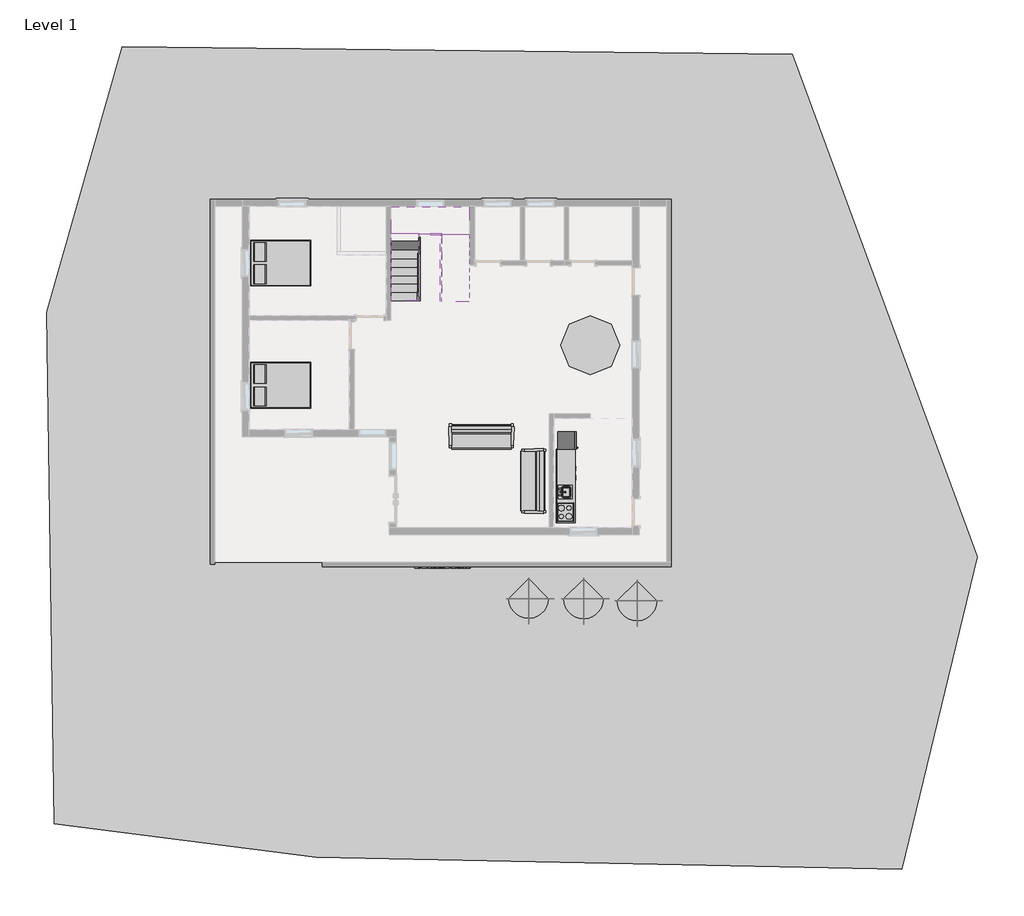
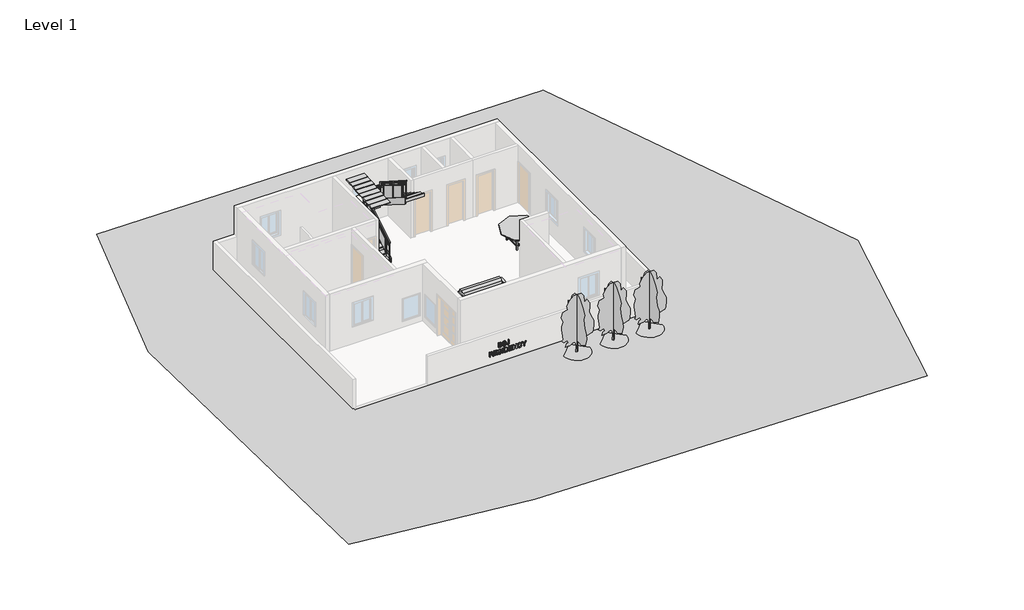
# One storey, part 2 of 2: 6 furniture elements, 6 proxies, 3 geographic elements, 3 members, 3 stair flights, 1 flow terminal, 1 railing, 1 slab.
"""IFC4 building model written with IfcOpenShell, lengths in millimetres."""

from ifc_helpers import new_model, si_unit, frame, origin, place, context, project, spatial, polyline, outline, extrude, faceted_brep, triangles, transform, mapped, element, save
from components import proxy_a6faaae8, proxy_45b28599, kitchenette_medium_kitchenette_medium_844211aa, proxy_c523a7b7, flow_terminal_871c2e40, furniture_1d2926bd, furniture_8d292e24, furniture_aff9b2fb, furniture_7cf74a4d, rpc_tree_deciduous_red_ash_25_5dd3353f, non_monolithic_landing_a2679692, stair_flight_49f3f953, stair_flight_b3fe96e5, stair_flight_42c3951d

model = new_model("IFC4")

# Units and contexts
model_context = context("Model", 3, world=origin())
ifc_project = project(units=[si_unit("LENGTHUNIT", "METRE", prefix="MILLI")], contexts=[model_context])

# Site, building, storey
site = spatial("IfcSite", under=ifc_project)
building = spatial("IfcBuilding", under=site)
storey = spatial("IfcBuildingStorey", under=building, Name="Level 1", Elevation=0.0)

# Proxies
placement = place(None, origin())
element("IfcBuildingElementProxy", 1, Name="Building Element Proxy", at=placement, inside=storey, context=model_context, shape_type="Tessellation", body=[
    triangles([(-16438.8070587, 19561.2664673, -152.4), (5929.6961975, 19305.9913513, -152.4), (12120.1241547, 2521.6364891, -152.4), (9599.2797684, -7912.7437592, -152.4), (-9961.1954681, -7497.921405, -152.4), (-18704.3757477, -6381.0919006, -152.4), (-18959.6520264, 10690.4486298, -152.4)], [[1, 7, 2], [5, 7, 6], [5, 4, 3], [3, 2, 5], [5, 2, 7]], closed=False),
])
element("IfcBuildingElementProxy", 2, Name="24\" Arial", ObjectType="24\" Arial", at=placement, inside=storey, context=model_context, shape_type="SweptSolid", body=[
    extrude(outline(polyline([(834.7006374, -6040.136942), (853.9637739, -6042.7239791), (870.1254059, -6050.4850902), (883.1855332, -6063.4202754), (893.1441559, -6081.5295346), (901.6806431, -6068.3591643), (913.0614012, -6058.9517569), (927.2864302, -6053.3073124), (944.35573, -6051.4258309), (970.4612855, -6056.9085856), (991.2751744, -6073.3568495), (1002.4317716, -6091.8629837), (1006.1506374, -6111.162868), (1006.1506374, -6216.9962013), (765.3210077, -6216.9962013), (765.3210077, -6099.6387939), (770.4362855, -6078.7367106), (785.7821188, -6059.6573124), (808.5950818, -6045.0170346), (834.7006374, -6040.136942)]), holes=[polyline([(939.8872114, -6081.411942), (925.0852438, -6084.4987476), (913.3700818, -6093.7591643), (906.7554985, -6105.3567337), (904.5506374, -6118.7475902), (904.5506374, -6186.8924976), (979.8098966, -6186.8924976), (979.8098966, -6131.7415717), (977.5168411, -6113.6176133), (970.6376744, -6098.2864791), (957.3938087, -6085.6305763), (939.8872114, -6081.411942)]), polyline([(835.6413781, -6070.2406457), (818.6786466, -6072.9232268), (804.4793411, -6080.9709698), (794.8661466, -6092.9139675), (791.6617485, -6107.2823124), (791.6617485, -6186.8924976), (878.2098966, -6186.8924976), (878.2098966, -6118.9827754), (875.5493642, -6097.6580937), (867.567767, -6082.4261782), (854.265105, -6073.2870288), (835.6413781, -6070.2406457)])]), frame((0.0, 2146.5230289, 0.0), z_axis=(0.0, 1.0, 0.0), x_axis=(0.0, 0.0, 1.0)), (0.0, 0.0, 1.0), 50.8),
    extrude(outline(polyline([(834.4066559, -5829.4110161), (854.1034151, -5832.4978217), (871.5659151, -5841.7582383), (884.427605, -5855.4136782), (892.0858225, -5872.3911087), (911.4886003, -5946.1216643), (916.4679117, -5959.2663113), (923.3507531, -5968.6553448), (932.1371246, -5974.288765), (942.8270262, -5976.1665717), (958.8343179, -5972.352162), (971.9311929, -5960.9089328), (980.6624429, -5943.9241527), (983.5728596, -5923.4850902), (980.8241327, -5900.436942), (972.5779522, -5882.6804606), (957.3056142, -5869.6129837), (936.0654522, -5864.3948124), (936.0654522, -5835.8198124), (966.7277207, -5842.12939), (978.7736119, -5849.3990008), (988.6293411, -5859.4118263), (1001.7703133, -5887.6671214), (1006.1506374, -5926.8952754), (1001.4763318, -5959.0862476), (987.4534151, -5984.3980532), (965.8310772, -6000.8022198), (938.3585077, -6006.2702754), (919.0145262, -6003.2790138), (903.4335077, -5994.3052291), (891.6154522, -5979.3489212), (883.5603596, -5958.4100902), (866.6858225, -5894.3221272), (861.1111987, -5879.0938865), (853.5007531, -5868.2165717), (843.8544857, -5861.6901828), (832.1723966, -5859.5147198), (814.4379637, -5863.3658772), (800.2754059, -5874.9193495), (790.9929406, -5892.7052291), (787.8987855, -5915.2536087), (791.2281258, -5945.7027407), (801.2161466, -5966.9649513), (818.5243063, -5980.0397777), (843.8140633, -5985.9267569), (843.8140633, -6013.7962013), (810.5574082, -6007.5196967), (797.1206171, -6000.1591353), (785.811517, -5989.9837013), (776.8469192, -5977.0742395), (770.443635, -5961.5115948), (765.3210077, -5922.4267569), (770.0908573, -5884.451699), (784.4004059, -5854.8404143), (794.6805708, -5843.7150526), (806.4416675, -5835.7683657), (819.6836958, -5831.0003535), (834.4066559, -5829.4110161)])), frame((0.0, 2146.5230289, 0.0), z_axis=(0.0, 1.0, 0.0), x_axis=(0.0, 0.0, 1.0)), (0.0, 0.0, 1.0), 50.8),
    extrude(outline(polyline([(823.70573, -5675.1295346), (1006.1506374, -5675.1295346), (1006.1506374, -5705.2332383), (833.0543411, -5705.2332383), (815.6432878, -5707.9011203), (802.5684614, -5715.9047661), (794.3884267, -5728.1123471), (791.6617485, -5743.3920346), (794.0944452, -5756.8563865), (801.3925355, -5767.4985161), (812.6593758, -5774.42178), (826.9983225, -5776.7295346), (848.1061929, -5776.7295346), (848.1061929, -5806.8332383), (821.3538781, -5806.8332383), (800.5105911, -5802.805692), (782.9011003, -5790.7230532), (769.7160309, -5769.6298819), (765.3210077, -5742.4512939), (766.8056142, -5725.7751944), (771.2594337, -5711.2010624), (778.6824661, -5698.7288981), (789.0747114, -5688.3587013), (806.052142, -5678.4368263), (823.70573, -5675.1295346)])), frame((0.0, 2146.5230289, 0.0), z_axis=(0.0, 1.0, 0.0), x_axis=(0.0, 0.0, 1.0)), (0.0, 0.0, 1.0), 50.8),
    extrude(outline(polyline([(407.8395262, -6475.1707383), (415.7770262, -6475.1707383), (424.861054, -6482.3144883), (436.2381374, -6485.5188865), (486.4501744, -6487.9295346), (507.6168411, -6493.2799976), (526.7844337, -6514.9758309), (538.5730911, -6501.49678), (551.4788781, -6491.8688865), (565.5017948, -6486.0921504), (580.6418411, -6484.1665717), (609.4373272, -6487.811942), (629.8543411, -6498.7480532), (638.0858225, -6508.8058946), (643.9654522, -6521.8109004), (648.6691559, -6556.662405), (648.6691559, -6664.7887939), (407.8395262, -6664.7887939), (407.8395262, -6634.6850902), (513.2024892, -6634.6850902), (513.2024892, -6554.8397198), (510.4243642, -6539.2219536), (502.0899892, -6527.881618), (488.1993642, -6520.8187129), (468.7524892, -6518.0332383), (430.7112855, -6517.0924976), (407.8395262, -6511.3304606), (407.8395262, -6475.1707383)]), holes=[polyline([(585.58073, -6514.2702754), (565.4393237, -6516.8132152), (551.052605, -6524.4420346), (542.4205737, -6537.1567337), (539.54323, -6554.9573124), (539.54323, -6634.6850902), (622.3284151, -6634.6850902), (622.3284151, -6555.2512939), (619.8883688, -6538.7368842), (612.56823, -6525.6473587), (600.9412624, -6517.1145462), (585.58073, -6514.2702754)])]), frame((0.0, 2146.5230289, 0.0), z_axis=(0.0, 1.0, 0.0), x_axis=(0.0, 0.0, 1.0)), (0.0, 0.0, 1.0), 50.8),
    extrude(outline(polyline([(407.8395262, -6265.9735161), (434.180267, -6265.9735161), (434.180267, -6405.1443495), (520.7284151, -6405.1443495), (520.7284151, -6276.674442), (547.0691559, -6276.674442), (547.0691559, -6405.1443495), (622.3284151, -6405.1443495), (622.3284151, -6271.500368), (648.6691559, -6271.500368), (648.6691559, -6435.2480532), (407.8395262, -6435.2480532), (407.8395262, -6265.9735161)])), frame((0.0, 2146.5230289, 0.0), z_axis=(0.0, 1.0, 0.0), x_axis=(0.0, 0.0, 1.0)), (0.0, 0.0, 1.0), 50.8),
    extrude(outline(polyline([(476.9251744, -6047.662868), (496.6219337, -6050.7496735), (514.0844337, -6060.0100902), (526.9461235, -6073.66553), (534.6043411, -6090.6429606), (554.0071188, -6164.3735161), (558.9864302, -6177.5181631), (565.8692716, -6186.9071967), (574.6556431, -6192.5406168), (585.3455448, -6194.4184235), (601.3528364, -6190.6040138), (614.4497114, -6179.1607846), (623.1809614, -6162.1760045), (626.0913781, -6141.736942), (623.3426512, -6118.6887939), (615.0964707, -6100.9323124), (599.8241327, -6087.8648356), (578.5839707, -6082.6466643), (578.5839707, -6054.0716643), (609.2462392, -6060.3812418), (621.2921304, -6067.6508526), (631.1478596, -6077.6636782), (644.2888318, -6105.9189733), (648.6691559, -6145.1471272), (643.9948503, -6177.3380995), (629.9719337, -6202.649905), (608.3495957, -6219.0540717), (580.8770262, -6224.5221272), (561.5330448, -6221.5308657), (545.9520262, -6212.5570809), (534.1339707, -6197.6007731), (526.0788781, -6176.661942), (509.2043411, -6112.5739791), (503.6297172, -6097.3457383), (496.0192716, -6086.4684235), (486.3730043, -6079.9420346), (474.6909151, -6077.7665717), (456.9564823, -6081.6177291), (442.7939244, -6093.1712013), (433.5114591, -6110.9570809), (430.417304, -6133.5054606), (433.7466443, -6163.9545925), (443.7346651, -6185.2168032), (461.0428249, -6198.2916295), (486.3325818, -6204.1786087), (486.3325818, -6232.0480532), (453.0759267, -6225.7715485), (439.6391356, -6218.4109872), (428.3300355, -6208.2355532), (419.3654377, -6195.3260913), (412.9621536, -6179.7634467), (407.8395262, -6140.6786087), (412.6093758, -6102.7035508), (426.9189244, -6073.0922661), (437.1990893, -6061.9669044), (448.960186, -6054.0202175), (462.2022143, -6049.2522054), (476.9251744, -6047.662868)])), frame((0.0, 2146.5230289, 0.0), z_axis=(0.0, 1.0, 0.0), x_axis=(0.0, 0.0, 1.0)), (0.0, 0.0, 1.0), 50.8),
    extrude(outline(polyline([(-5972.4036087, 2146.5230289), (-6002.5073124, 2146.5230289), (-6002.5073124, 2197.3230289), (-5972.4036087, 2197.3230289), (-5972.4036087, 2146.5230289)])), frame((0.0, 0.0, 407.8395262), z_axis=(0.0, 0.0, 1.0), x_axis=(1.0, 0.0, 0.0)), (0.0, 0.0, 1.0), 240.8296296),
    extrude(outline(polyline([(530.429804, -5727.8110161), (558.3286466, -5729.8247893), (582.9348966, -5735.8661087), (604.248554, -5745.9349745), (622.2696188, -5760.0313865), (633.8194163, -5773.5214617), (642.0692716, -5787.9449282), (647.0191848, -5803.3017858), (648.6691559, -5819.5920346), (648.6691559, -5915.9591643), (407.8395262, -5915.9591643), (407.8395262, -5812.4188865), (409.8202265, -5797.3045636), (415.7623272, -5782.8884467), (425.6658283, -5769.1705358), (439.53073, -5756.1508309), (458.7277207, -5743.752162), (480.2765633, -5734.8959698), (504.1772577, -5729.5822545), (530.429804, -5727.8110161)]), holes=[polyline([(530.429804, -5757.9147198), (491.5801512, -5761.6923819), (461.2265633, -5773.025368), (449.3938087, -5781.6169768), (440.9418411, -5791.693192), (435.8706605, -5803.2540138), (434.180267, -5816.299442), (434.180267, -5885.8554606), (622.3284151, -5885.8554606), (622.3284151, -5824.5309235), (616.5663781, -5797.2053448), (609.3638318, -5785.9348298), (599.280267, -5776.2591643), (569.8674198, -5762.5008309), (530.429804, -5757.9147198)])]), frame((0.0, 2146.5230289, 0.0), z_axis=(0.0, 1.0, 0.0), x_axis=(0.0, 0.0, 1.0)), (0.0, 0.0, 1.0), 50.8),
    extrude(outline(polyline([(407.8395262, -5513.3809235), (434.180267, -5513.3809235), (434.180267, -5652.5517569), (520.7284151, -5652.5517569), (520.7284151, -5524.0818495), (547.0691559, -5524.0818495), (547.0691559, -5652.5517569), (622.3284151, -5652.5517569), (622.3284151, -5518.9077754), (648.6691559, -5518.9077754), (648.6691559, -5682.6554606), (407.8395262, -5682.6554606), (407.8395262, -5513.3809235)])), frame((0.0, 2146.5230289, 0.0), z_axis=(0.0, 1.0, 0.0), x_axis=(0.0, 0.0, 1.0)), (0.0, 0.0, 1.0), 50.8),
    extrude(outline(polyline([(407.8395262, -5287.5443495), (648.6691559, -5287.5443495), (648.6691559, -5317.6480532), (457.5811929, -5317.6480532), (648.6691559, -5432.4772198), (648.6691559, -5471.9295346), (407.8395262, -5471.9295346), (407.8395262, -5441.8258309), (599.9270262, -5441.8258309), (407.8395262, -5322.0577754), (407.8395262, -5287.5443495)])), frame((0.0, 2146.5230289, 0.0), z_axis=(0.0, 1.0, 0.0), x_axis=(0.0, 0.0, 1.0)), (0.0, 0.0, 1.0), 50.8),
    extrude(outline(polyline([(498.0330448, -5042.2462013), (498.0330448, -5073.4670346), (470.0974545, -5083.7784351), (450.1434614, -5098.7200439), (438.1710656, -5118.291861), (434.180267, -5142.4938865), (435.7879782, -5158.1447256), (440.6111119, -5172.2301133), (448.649668, -5184.7500497), (459.9036466, -5195.7045346), (489.3826397, -5210.9621735), (526.3728596, -5216.0480532), (565.5973387, -5211.0871157), (581.951896, -5204.8859438), (596.1346651, -5196.2043032), (607.5944308, -5185.4684669), (615.7799776, -5173.1047082), (620.6913058, -5159.1130271), (622.3284151, -5143.4934235), (619.3518526, -5122.4847719), (610.4221651, -5104.7319652), (595.5393526, -5090.2350034), (574.7034151, -5078.9938865), (574.7034151, -5047.1262939), (606.4754637, -5062.3104374), (629.7073503, -5083.8739791), (643.9287045, -5110.6850902), (648.6691559, -5141.611942), (646.3981489, -5165.3362476), (639.5851281, -5186.3559235), (628.2300934, -5204.6709698), (612.3330448, -5220.2813865), (594.6022867, -5231.5996735), (574.6299198, -5239.6841643), (552.4159441, -5244.5348587), (527.9603596, -5246.1517569), (502.2314678, -5244.3621446), (479.137385, -5238.9933078), (458.6781113, -5230.0452464), (440.8536466, -5217.5179606), (426.409969, -5202.0545346), (416.0930563, -5184.2980532), (409.9029088, -5164.2485161), (407.8395262, -5141.9059235), (413.4766212, -5106.4407326), (420.5229898, -5091.3457022), (430.3879059, -5078.0090485), (458.5733804, -5056.6108714), (498.0330448, -5042.2462013)])), frame((0.0, 2146.5230289, 0.0), z_axis=(0.0, 1.0, 0.0), x_axis=(0.0, 0.0, 1.0)), (0.0, 0.0, 1.0), 50.8),
    extrude(outline(polyline([(648.6691559, -4814.4693495), (648.6691559, -4849.8059235), (531.4881374, -4917.774442), (648.6691559, -4986.624905), (648.6691559, -5024.136942), (502.3251744, -4933.8258309), (407.8395262, -4933.8258309), (407.8395262, -4903.7221272), (504.1478596, -4903.7221272), (648.6691559, -4814.4693495)])), frame((0.0, 2146.5230289, 0.0), z_axis=(0.0, 1.0, 0.0), x_axis=(0.0, 0.0, 1.0)), (0.0, 0.0, 1.0), 50.8),
])
proxy_shape = proxy_a6faaae8(model_context)
element("IfcBuildingElementProxy", 3, Name="Cook Top-4 Unit2 : 22\" x 20\"", ObjectType="Cook Top-4 Unit2 : 22\" x 20\"", at=placement, inside=storey, context=model_context, shape_type="MappedRepresentation", body=[
    mapped(proxy_shape, transform((-1644.6867944, 4013.4230289, 0.0), x_axis=(0.0, 1.0000000000000009, 0.0), y_axis=(-1.0000000000000009, 0.0, 0.0), z_axis=(0.0, 0.0, 1.0))),
])
proxy_2_shape = proxy_45b28599(model_context)
element("IfcBuildingElementProxy", 4, Name="Dishwasher : 24\" x 24\" x 34\"", ObjectType="Dishwasher : 24\" x 24\" x 34\"", at=placement, inside=storey, context=model_context, shape_type="MappedRepresentation", body=[
    mapped(proxy_2_shape, transform((-1352.8372296, 4964.6055604, 0.0), x_axis=(0.0, 1.0000000000000009, 0.0), y_axis=(-1.0000000000000009, 0.0, 0.0), z_axis=(0.0, 0.0, 1.0))),
])
kitchenette_medium_kitchenette_medium_shape = kitchenette_medium_kitchenette_medium_844211aa(model_context)
element("IfcBuildingElementProxy", 5, Name="Kitchenette - Medium : Kitchenette - Medium", ObjectType="Kitchenette - Medium : Kitchenette - Medium", at=placement, inside=storey, context=model_context, shape_type="MappedRepresentation", body=[
    mapped(kitchenette_medium_kitchenette_medium_shape, transform((-1949.4867944, 4337.585324, 0.0), x_axis=(0.0, 1.0000000000000009, 0.0), y_axis=(-1.0000000000000009, 0.0, 0.0), z_axis=(0.0, 0.0, 1.0))),
])
proxy_3_shape = proxy_c523a7b7(model_context)
element("IfcBuildingElementProxy", 6, Name="Refrigerator : 24\" x 25\" LH", ObjectType="Refrigerator : 24\" x 25\" LH", at=placement, inside=storey, context=model_context, shape_type="MappedRepresentation", body=[
    mapped(proxy_3_shape, transform((-1599.0378229, 6407.3730289, 0.0), x_axis=(0.0, 1.0000000000000009, 0.0), y_axis=(-1.0000000000000009, 0.0, 0.0), z_axis=(0.0, 0.0, 1.0))),
])

# Flow terminal
flow_terminal_shape = flow_terminal_871c2e40(model_context)
element("IfcFlowTerminal", 7, ObjectType="Sink Kitchen-Island : 18\" x 18\"", at=placement, inside=storey, context=model_context, shape_type="MappedRepresentation", body=[
    mapped(flow_terminal_shape, transform((-1642.3413933, 4670.8337884, -14.4), x_axis=(0.0, 1.0000000000000009, 0.0), y_axis=(-1.0000000000000009, 0.0, 0.0), z_axis=(0.0, 0.0, 1.0))),
])

# Furniture
furniture_shape = furniture_1d2926bd(model_context)
element("IfcFurniture", 8, ObjectType="Bed-Box : Queen 60\" x 79\"", at=placement, inside=storey, context=model_context, shape_type="MappedRepresentation", body=[
    mapped(furniture_shape, transform((-11378.7163026, 7916.0705699, 0.0), x_axis=(0.0, 1.0000000000000002, 0.0), y_axis=(-1.0000000000000002, 0.0, 0.0), z_axis=(0.0, 0.0, 1.0))),
])
element("IfcFurniture", 9, ObjectType="Bed-Box : Queen 60\" x 79\"", at=placement, inside=storey, context=model_context, shape_type="MappedRepresentation", body=[
    mapped(furniture_shape, transform((-11378.7163026, 11992.7705699, 0.0), x_axis=(0.0, 1.0000000000000002, 0.0), y_axis=(-1.0000000000000002, 0.0, 0.0), z_axis=(0.0, 0.0, 1.0))),
])
furniture_2_shape = furniture_8d292e24(model_context)
element("IfcFurniture", 10, ObjectType="Counter Top w Sink Hole : 24\" Depth", at=placement, inside=storey, context=model_context, shape_type="MappedRepresentation", body=[
    mapped(furniture_2_shape, transform((-1949.4867944, 4870.985324, -14.4), x_axis=(0.0, 1.0000000000000009, 0.0), y_axis=(-1.0000000000000009, 0.0, 0.0), z_axis=(0.0, 0.0, 1.0))),
])
furniture_3_shape = furniture_aff9b2fb(model_context)
element("IfcFurniture", 11, ObjectType="Sofa-Pensi : 84\"", at=placement, inside=storey, context=model_context, shape_type="MappedRepresentation", body=[
    mapped(furniture_3_shape, transform((-4719.9800439, 6263.6131929, 0.0), x_axis=(1.0, 0.0, 0.0), y_axis=(0.0, 1.0, 0.0), z_axis=(0.0, 0.0, 1.0))),
])
element("IfcFurniture", 12, ObjectType="Sofa-Pensi : 84\"", at=placement, inside=storey, context=model_context, shape_type="MappedRepresentation", body=[
    mapped(furniture_3_shape, transform((-2988.5966305, 5333.4292789, 0.0), x_axis=(0.0, -1.0000000000000002, 0.0), y_axis=(1.0000000000000002, 0.0, 0.0), z_axis=(0.0, 0.0, 1.0))),
])
furniture_4_shape = furniture_7cf74a4d(model_context)
element("IfcFurniture", 13, ObjectType="Table-Dining Round w Chairs : 60\" Diameter", at=placement, inside=storey, context=model_context, shape_type="MappedRepresentation", body=[
    mapped(furniture_4_shape, transform((-910.1687616, 9773.6017175, 0.0), x_axis=(1.0, 0.0, 0.0), y_axis=(0.0, 1.0, 0.0), z_axis=(0.0, 0.0, 1.0))),
])

# Geographic elements
rpc_tree_deciduous_red_ash_25_shape = rpc_tree_deciduous_red_ash_25_5dd3353f(model_context)
element("IfcGeographicElement", 14, ObjectType="RPC Tree - Deciduous : Red Ash - 25'", at=placement, inside=storey, context=model_context, shape_type="MappedRepresentation", body=[
    mapped(rpc_tree_deciduous_red_ash_25_shape, transform((-2863.8867944, 1130.5230289, 0.0), x_axis=(1.0, 0.0, 0.0), y_axis=(0.0, 1.0, 0.0), z_axis=(0.0, 0.0, 1.0))),
])
element("IfcGeographicElement", 15, ObjectType="RPC Tree - Deciduous : Red Ash - 25'", at=placement, inside=storey, context=model_context, shape_type="MappedRepresentation", body=[
    mapped(rpc_tree_deciduous_red_ash_25_shape, transform((755.6132056, 1054.3230289, 0.0), x_axis=(1.0, 0.0, 0.0), y_axis=(0.0, 1.0, 0.0), z_axis=(0.0, 0.0, 1.0))),
])
element("IfcGeographicElement", 16, ObjectType="RPC Tree - Deciduous : Red Ash - 25'", at=placement, inside=storey, context=model_context, shape_type="MappedRepresentation", body=[
    mapped(rpc_tree_deciduous_red_ash_25_shape, transform((-1030.0266382, 1118.9211458, 0.0), x_axis=(1.0, 0.0, 0.0), y_axis=(0.0, 1.0, 0.0), z_axis=(0.0, 0.0, 1.0))),
])

# Members
element("IfcMember", 17, ObjectType="Stringer - 2\" Width", at=placement, inside=storey, context=model_context, shape_type="SweptSolid", body=[
    extrude(outline(polyline([(11074.6230289, 0.0), (11074.6230289, 215.0106437), (13259.0230289, 1605.083371), (13259.0230289, 1243.8010268), (11304.4785583, 0.0), (11074.6230289, 0.0)])), frame((-6534.1867944, 0.0, 0.0), z_axis=(1.0, 0.0, 0.0), x_axis=(0.0, 1.0, 0.0)), (0.0, 0.0, 1.0), 50.8),
])
element("IfcMember", 18, ObjectType="Stringer - 2\" Width", at=placement, inside=storey, context=model_context, shape_type="SweptSolid", body=[
    extrude(outline(polyline([(13259.0230289, 1841.3136224), (13259.0230289, 1480.0312782), (11064.8419954, 2876.3282995), (11064.8419954, 3237.6106437), (13259.0230289, 1841.3136224)])), frame((-5812.9737939, 0.0, 0.0), z_axis=(1.0, 0.0, 0.0), x_axis=(0.0, 1.0, 0.0)), (0.0, 0.0, 1.0), 50.8),
])
element("IfcMember", 19, ObjectType="Stringer - 2\" Width", at=placement, inside=storey, context=model_context, shape_type="SweptSolid", body=[
    extrude(outline(polyline([(-6534.1867944, 13259.0230289), (-6534.1867944, 13309.8230289), (-5762.1737939, 13309.8230289), (-5762.1737939, 13259.0230289), (-6534.1867944, 13259.0230289)])), frame((0.0, 0.0, 1371.6), z_axis=(0.0, 0.0, 1.0), x_axis=(1.0, 0.0, 0.0)), (0.0, 0.0, 1.0), 304.8),
])

# Railing
element("IfcRailing", 20, ObjectType="Glass Panel - Bottom Fill", at=placement, inside=storey, context=model_context, shape_type="SolidModel", body=[
    faceted_brep([(-6584.9867944, 11074.6230289, 1092.2), (-6584.9867944, 11074.6230289, 1031.986276), (-6534.1867944, 11074.6230289, 1031.986276), (-6534.1867944, 11074.6230289, 1092.2), (-5711.3737939, 11064.8419954, 4114.8), (-5762.1737939, 11064.8419954, 4114.8), (-5762.1737939, 11064.8419954, 4054.586276), (-5711.3737939, 11064.8419954, 4054.586276), (-6534.1867944, 13284.4230289, 2438.2226396), (-6534.1867944, 13233.6230289, 2466.1090909), (-6584.9867944, 13233.6230289, 2466.1090909), (-6457.9867944, 13309.8230289, 2514.6), (-6457.9867944, 13309.8230289, 2463.8), (-5762.1737939, 13309.8230289, 2463.8), (-5762.1737939, 13309.8230289, 2514.6), (-6457.9867944, 13360.6230289, 2514.6), (-5711.3737939, 13360.6230289, 2514.6), (-5762.1737939, 13300.0419954, 2692.4), (-5762.1737939, 13249.2419954, 2664.5135487), (-5711.3737939, 13300.0419954, 2692.4), (-6584.9867944, 13284.4230289, 2438.2226396), (-6584.9867944, 13233.6230289, 2514.6), (-6584.9867944, 13284.4230289, 2463.8), (-6534.1867944, 13284.4230289, 2463.8), (-6534.1867944, 13233.6230289, 2514.6), (-6584.9867944, 13360.6230289, 2514.6), (-6584.9867944, 13360.6230289, 2463.8), (-6534.1867944, 13309.8230289, 2463.8), (-6534.1867944, 13309.8230289, 2514.6), (-6457.9867944, 13360.6230289, 2463.8), (-5711.3737939, 13360.6230289, 2463.8), (-5711.3737939, 13300.0419954, 2514.6), (-5711.3737939, 13249.2419954, 2463.8), (-5762.1737939, 13249.2419954, 2463.8), (-5762.1737939, 13300.0419954, 2514.6), (-5711.3737939, 13249.2419954, 2664.5135487)], [[[0, 1, 2, 3]], [[4, 5, 6, 7]], [[3, 2, 8, 9]], [[0, 3, 9, 10]], [[11, 12, 13, 14]], [[15, 11, 14, 16]], [[17, 18, 6, 5]], [[19, 17, 5, 4]], [[1, 0, 10, 20]], [[2, 1, 20, 8]], [[20, 10, 21, 22]], [[8, 20, 22, 23]], [[9, 8, 23, 24]], [[10, 9, 24, 21]], [[22, 21, 25, 26]], [[23, 22, 26, 27]], [[24, 23, 27, 28]], [[21, 24, 28, 25]], [[26, 25, 15, 29]], [[27, 26, 29, 12]], [[28, 27, 12, 11]], [[25, 28, 11, 15]], [[29, 15, 16, 30]], [[12, 29, 30, 13]], [[30, 16, 31, 32]], [[13, 30, 32, 33]], [[14, 13, 33, 34]], [[16, 14, 34, 31]], [[32, 31, 19, 35]], [[33, 32, 35, 18]], [[34, 33, 18, 17]], [[31, 34, 17, 19]], [[35, 19, 4, 7]], [[18, 35, 7, 6]]]),
    faceted_brep([(-6546.8867944, 11074.6230289, 1005.653431), (-6572.2867944, 11074.6230289, 1005.653431), (-6572.2867944, 11074.6230289, 975.546569), (-6546.8867944, 11074.6230289, 975.546569), (-6546.8867944, 13317.6902093, 2433.0598185), (-6546.8867944, 13331.3268468, 2411.6308167), (-6572.2867944, 13352.7558486, 2425.2674542), (-6572.2867944, 13339.1192111, 2446.696456)], [[[0, 1, 2, 3]], [[4, 5, 6, 7]], [[1, 0, 4, 7]], [[2, 1, 7, 6]], [[3, 2, 6, 5]], [[0, 3, 5, 4]]]),
    faceted_brep([(-6555.6906123, 13322.5230289, 2425.7), (-6577.1196141, 13347.9230289, 2425.7), (-6563.4829766, 13347.9230289, 2400.3), (-6542.0539748, 13322.5230289, 2400.3), (-5749.4737939, 13322.5230289, 2425.7), (-5749.4737939, 13322.5230289, 2400.3), (-5724.0737939, 13347.9230289, 2400.3), (-5724.0737939, 13347.9230289, 2425.7)], [[[0, 1, 2, 3]], [[4, 5, 6, 7]], [[1, 0, 4, 7]], [[2, 1, 7, 6]], [[3, 2, 6, 5]], [[0, 3, 5, 4]]]),
    faceted_brep([(-5749.4737939, 13303.7402441, 2603.5), (-5724.0737939, 13303.7402441, 2603.5), (-5724.0737939, 13296.3437467, 2578.1), (-5749.4737939, 13296.3437467, 2578.1), (-5749.4737939, 11064.8419954, 4028.253431), (-5749.4737939, 11064.8419954, 3998.146569), (-5724.0737939, 11064.8419954, 3998.146569), (-5724.0737939, 11064.8419954, 4028.253431)], [[[0, 1, 2, 3]], [[4, 5, 6, 7]], [[1, 0, 4, 7]], [[2, 1, 7, 6]], [[3, 2, 6, 5]], [[0, 3, 5, 4]]]),
    faceted_brep([(-6546.8867944, 11074.6230289, 904.053431), (-6572.2867944, 11074.6230289, 904.053431), (-6572.2867944, 11074.6230289, 873.946569), (-6546.8867944, 11074.6230289, 873.946569), (-6546.8867944, 13317.6902093, 2331.4598185), (-6546.8867944, 13331.3268468, 2310.0308167), (-6572.2867944, 13352.7558486, 2323.6674542), (-6572.2867944, 13339.1192111, 2345.096456)], [[[0, 1, 2, 3]], [[4, 5, 6, 7]], [[1, 0, 4, 7]], [[2, 1, 7, 6]], [[3, 2, 6, 5]], [[0, 3, 5, 4]]]),
    faceted_brep([(-6555.6906123, 13322.5230289, 2324.1), (-6577.1196141, 13347.9230289, 2324.1), (-6563.4829766, 13347.9230289, 2298.7), (-6542.0539748, 13322.5230289, 2298.7), (-5749.4737939, 13322.5230289, 2324.1), (-5749.4737939, 13322.5230289, 2298.7), (-5724.0737939, 13347.9230289, 2298.7), (-5724.0737939, 13347.9230289, 2324.1)], [[[0, 1, 2, 3]], [[4, 5, 6, 7]], [[1, 0, 4, 7]], [[2, 1, 7, 6]], [[3, 2, 6, 5]], [[0, 3, 5, 4]]]),
    faceted_brep([(-5749.4737939, 13303.7402441, 2501.9), (-5724.0737939, 13303.7402441, 2501.9), (-5724.0737939, 13296.3437467, 2476.5), (-5749.4737939, 13296.3437467, 2476.5), (-5749.4737939, 11064.8419954, 3926.653431), (-5749.4737939, 11064.8419954, 3896.546569), (-5724.0737939, 11064.8419954, 3896.546569), (-5724.0737939, 11064.8419954, 3926.653431)], [[[0, 1, 2, 3]], [[4, 5, 6, 7]], [[1, 0, 4, 7]], [[2, 1, 7, 6]], [[3, 2, 6, 5]], [[0, 3, 5, 4]]]),
    faceted_brep([(-5749.4737939, 13322.5230289, 2425.7), (-5724.0737939, 13347.9230289, 2425.7), (-5724.0737939, 13347.9230289, 2400.3), (-5749.4737939, 13322.5230289, 2400.3), (-5749.4737939, 13303.7402441, 2425.7), (-5749.4737939, 13296.3437467, 2400.3), (-5724.0737939, 13296.3437467, 2400.3), (-5724.0737939, 13303.7402441, 2425.7)], [[[0, 1, 2, 3]], [[4, 5, 6, 7]], [[1, 0, 4, 7]], [[2, 1, 7, 6]], [[3, 2, 6, 5]], [[0, 3, 5, 4]]]),
    faceted_brep([(-5749.4737939, 13322.5230289, 2324.1), (-5724.0737939, 13347.9230289, 2324.1), (-5724.0737939, 13347.9230289, 2298.7), (-5749.4737939, 13322.5230289, 2298.7), (-5749.4737939, 13303.7402441, 2324.1), (-5749.4737939, 13296.3437467, 2298.7), (-5724.0737939, 13296.3437467, 2298.7), (-5724.0737939, 13303.7402441, 2324.1)], [[[0, 1, 2, 3]], [[4, 5, 6, 7]], [[1, 0, 4, 7]], [[2, 1, 7, 6]], [[3, 2, 6, 5]], [[0, 3, 5, 4]]]),
    extrude(outline(polyline([(11363.2919954, 3808.2238417), (11375.9919954, 3800.1420235), (11375.9919954, 2844.8), (11363.2919954, 2844.8), (11363.2919954, 3808.2238417)])), frame((-5762.1737939, 0.0, 0.0), z_axis=(1.0, 0.0, 0.0), x_axis=(0.0, 1.0, 0.0)), (0.0, 0.0, 1.0), 50.8),
    extrude(outline(polyline([(12182.4419954, 2509.9818182), (11369.6419954, 3027.2181818), (11369.6419954, 3702.5829326), (12182.4419954, 3185.346569), (12182.4419954, 2509.9818182)])), frame((-5736.5886369, 0.0, 0.0), z_axis=(1.0, 0.0, 0.0), x_axis=(0.0, 1.0, 0.0)), (0.0, 0.0, 1.0), 6.35),
    extrude(outline(polyline([(12176.0919954, 3290.9874781), (12188.7919954, 3282.9056599), (12188.7919954, 2489.2), (12176.0919954, 2489.2), (12176.0919954, 3290.9874781)])), frame((-5762.1737939, 0.0, 0.0), z_axis=(1.0, 0.0, 0.0), x_axis=(0.0, 1.0, 0.0)), (0.0, 0.0, 1.0), 50.8),
    extrude(outline(polyline([(12995.2419954, 1976.5818182), (12182.4419954, 2493.8181818), (12182.4419954, 3185.346569), (12995.2419954, 2668.1102054), (12995.2419954, 1976.5818182)])), frame((-5736.5886369, 0.0, 0.0), z_axis=(1.0, 0.0, 0.0), x_axis=(0.0, 1.0, 0.0)), (0.0, 0.0, 1.0), 6.35),
    extrude(outline(polyline([(12988.8919954, 2773.7511144), (13001.5919954, 2765.6692963), (13001.5919954, 1955.8), (12988.8919954, 1955.8), (12988.8919954, 2773.7511144)])), frame((-5762.1737939, 0.0, 0.0), z_axis=(1.0, 0.0, 0.0), x_axis=(0.0, 1.0, 0.0)), (0.0, 0.0, 1.0), 50.8),
    extrude(outline(polyline([(-5748.1302942, 13309.8230289), (-5748.1302942, 13360.6230289), (-5735.4302942, 13360.6230289), (-5735.4302942, 13309.8230289), (-5748.1302942, 13309.8230289)])), frame((0.0, 0.0, 1600.2), z_axis=(0.0, 0.0, 1.0), x_axis=(1.0, 0.0, 0.0)), (0.0, 0.0, 1.0), 800.1),
    extrude(outline(polyline([(-6554.5802942, 13341.7581859), (-5741.7802942, 13341.7581859), (-5741.7802942, 13335.4081859), (-6554.5802942, 13335.4081859), (-6554.5802942, 13341.7581859)])), frame((0.0, 0.0, 1701.8), z_axis=(0.0, 0.0, 1.0), x_axis=(1.0, 0.0, 0.0)), (0.0, 0.0, 1.0), 596.9),
    extrude(outline(polyline([(-6560.9302942, 13309.8230289), (-6560.9302942, 13360.6230289), (-6548.2302942, 13360.6230289), (-6548.2302942, 13309.8230289), (-6560.9302942, 13309.8230289)])), frame((0.0, 0.0, 1600.2), z_axis=(0.0, 0.0, 1.0), x_axis=(1.0, 0.0, 0.0)), (0.0, 0.0, 1.0), 800.1),
    extrude(outline(polyline([(13011.3730289, 2208.0238417), (13024.0730289, 2216.1056599), (13024.0730289, 1244.6), (13011.3730289, 1244.6), (13011.3730289, 2208.0238417)])), frame((-6584.9867944, 0.0, 0.0), z_axis=(1.0, 0.0, 0.0), x_axis=(0.0, 1.0, 0.0)), (0.0, 0.0, 1.0), 50.8),
    extrude(outline(polyline([(12204.9230289, 909.7818182), (12204.9230289, 1593.2283872), (13017.7230289, 2110.4647508), (13017.7230289, 1427.0181818), (12204.9230289, 909.7818182)])), frame((-6566.1219514, 0.0, 0.0), z_axis=(1.0, 0.0, 0.0), x_axis=(0.0, 1.0, 0.0)), (0.0, 0.0, 1.0), 6.35),
    extrude(outline(polyline([(12198.5730289, 1690.7874781), (12211.2730289, 1698.8692963), (12211.2730289, 889.0), (12198.5730289, 889.0), (12198.5730289, 1690.7874781)])), frame((-6584.9867944, 0.0, 0.0), z_axis=(1.0, 0.0, 0.0), x_axis=(0.0, 1.0, 0.0)), (0.0, 0.0, 1.0), 50.8),
    extrude(outline(polyline([(11392.1230289, 376.3818182), (11392.1230289, 1075.9920235), (12204.9230289, 1593.2283872), (12204.9230289, 893.6181818), (11392.1230289, 376.3818182)])), frame((-6566.1219514, 0.0, 0.0), z_axis=(1.0, 0.0, 0.0), x_axis=(0.0, 1.0, 0.0)), (0.0, 0.0, 1.0), 6.35),
    extrude(outline(polyline([(11385.7730289, 1173.5511144), (11398.4730289, 1181.6329326), (11398.4730289, 355.6), (11385.7730289, 355.6), (11385.7730289, 1173.5511144)])), frame((-6584.9867944, 0.0, 0.0), z_axis=(1.0, 0.0, 0.0), x_axis=(0.0, 1.0, 0.0)), (0.0, 0.0, 1.0), 50.8),
    extrude(outline(polyline([(-5746.2987939, 13309.5669954), (-5727.2487939, 13309.5669954), (-5727.2487939, 13290.5169954), (-5746.2987939, 13290.5169954), (-5746.2987939, 13309.5669954)])), frame((0.0, 0.0, 1778.0), z_axis=(0.0, 0.0, 1.0), x_axis=(1.0, 0.0, 0.0)), (0.0, 0.0, 1.0), 685.8),
    extrude(outline(polyline([(-5746.2987939, 13325.6980289), (-5746.2987939, 13344.7480289), (-5727.2487939, 13344.7480289), (-5727.2487939, 13325.6980289), (-5746.2987939, 13325.6980289)])), frame((0.0, 0.0, 1600.2), z_axis=(0.0, 0.0, 1.0), x_axis=(1.0, 0.0, 0.0)), (0.0, 0.0, 1.0), 863.6),
    extrude(outline(polyline([(-6550.0617944, 13325.6980289), (-6569.1117944, 13325.6980289), (-6569.1117944, 13344.7480289), (-6550.0617944, 13344.7480289), (-6550.0617944, 13325.6980289)])), frame((0.0, 0.0, 1600.2), z_axis=(0.0, 0.0, 1.0), x_axis=(1.0, 0.0, 0.0)), (0.0, 0.0, 1.0), 863.6),
    extrude(outline(polyline([(11058.4919954, 4058.6271851), (11077.5419954, 4046.5044578), (11077.5419954, 3022.6), (11058.4919954, 3022.6), (11058.4919954, 4058.6271851)])), frame((-5746.2987939, 0.0, 0.0), z_axis=(1.0, 0.0, 0.0), x_axis=(0.0, 1.0, 0.0)), (0.0, 0.0, 1.0), 19.05),
    extrude(outline(polyline([(11068.2730289, 1027.9453669), (11087.3230289, 1040.0680941), (11087.3230289, 177.8), (11068.2730289, 177.8), (11068.2730289, 1027.9453669)])), frame((-6569.1117944, 0.0, 0.0), z_axis=(1.0, 0.0, 0.0), x_axis=(0.0, 1.0, 0.0)), (0.0, 0.0, 1.0), 19.05),
])

# Slab
non_monolithic_landing_shape = non_monolithic_landing_a2679692(model_context)
element("IfcSlab", 21, ObjectType="Non-Monolithic Landing", at=placement, inside=storey, context=model_context, shape_type="MappedRepresentation", body=[
    mapped(non_monolithic_landing_shape, transform((0.0, 0.0, 0.0), x_axis=(1.0, 0.0, 0.0), y_axis=(0.0, 1.0, 0.0), z_axis=(0.0, 0.0, 1.0))),
])

# Stair flights
stair_flight_shape = stair_flight_49f3f953(model_context)
element("IfcStairFlight", 22, ObjectType="2\" Tread 1\" Nosing 1/4\" Riser", at=placement, inside=storey, context=model_context, shape_type="MappedRepresentation", body=[
    mapped(stair_flight_shape, transform((0.0, 0.0, 0.0), x_axis=(1.0, 0.0, 0.0), y_axis=(0.0, 1.0, 0.0), z_axis=(0.0, 0.0, 1.0))),
])
stair_flight_2_shape = stair_flight_b3fe96e5(model_context)
element("IfcStairFlight", 23, ObjectType="2\" Tread 1\" Nosing 1/4\" Riser", at=placement, inside=storey, context=model_context, shape_type="MappedRepresentation", body=[
    mapped(stair_flight_2_shape, transform((0.0, 0.0, 0.0), x_axis=(1.0, 0.0, 0.0), y_axis=(0.0, 1.0, 0.0), z_axis=(0.0, 0.0, 1.0))),
])
stair_flight_3_shape = stair_flight_42c3951d(model_context)
element("IfcStairFlight", 24, ObjectType="2\" Tread 1\" Nosing 1/4\" Riser", at=placement, inside=storey, context=model_context, shape_type="MappedRepresentation", body=[
    mapped(stair_flight_3_shape, transform((0.0, 0.0, 0.0), x_axis=(1.0, 0.0, 0.0), y_axis=(0.0, 1.0, 0.0), z_axis=(0.0, 0.0, 1.0))),
])

save(model, "model.ifc")

# Revit data of these elements
# Type "Cook Top-4 Unit2 : 22\" x 20\""
#   Depth = 1' - 8"
#   Width = 1' - 10"
#   Burner Material = Steel, Chrome Plated
#   Cooktop Material = Steel, Polished
#   Default Elevation = 0
#   Assembly Code = ""
# Type "Dishwasher : 24\" x 24\" x 34\""
#   Label = "DW"
#   Assembly Code = "E1090400"
#   Depth = 2' - 0"
#   Height = 2' - 10"
#   Width = 2' - 0"
#   Dishwasher Material = Steel, Paint Finish, Ivory, Glossy
#   Panel Face Material = Plastic, Opaque Black
#   Default Elevation = 0
# Type "Kitchenette - Medium : Kitchenette - Medium"
#   Assembly Code = "E1090400"
#   Counter Length = 8' - 0"
#   Cabinet Width = 4' - 6"
#   Cabinet Height = 2' - 10 1/2"
#   Cabinet Depth = 2' - 0"
#   Toe Depth = 0' - 3"
#   Toe Height = 0' - 3 1/2"
#   Cabinet Material = Cabinets
#   Door/Drawer Material = Cabinets
#   Handle Material = Cabinets - Handles
#   Default Elevation = 0
# Type "Refrigerator : 24\" x 25\" LH"
#   Label = "REF."
#   Assembly Code = "E1090400"
#   Depth = 2' - 0 3/4"
#   Handle = 0' - 1 1/2"
#   Height = 5' - 3 1/2"
#   Rear Clearance = 0' - 2"
#   Top Door Height = 1' - 8"
#   Width = 1' - 11 1/2"
#   Material = Steel, Paint Finish, Ivory, Glossy
#   Default Elevation = 0
# Type "Sink Kitchen-Island : 18\" x 18\""
#   Assembly Code = "D2010410"
#   Counter Height = 3' - 0"
#   Depth = 1' - 6"
#   Width = 1' - 6"
#   Faucet Material = Steel, Polished
#   Sink Material = Steel, Polished
#   Default Elevation = 0
# Type "Bed-Box : Queen 60\" x 79\""
#   Assembly Code = "E2020200"
#   Length = 6' - 7"
#   Width = 5' - 0"
#   Frame Material = Birch
#   Mattress Material = Linen, White
#   Default Elevation = 0
# Type "Counter Top w Sink Hole : 24\" Depth"
#   Assembly Code = "C1030400"
#   Counter Thickness = 0' - 1 1/2"
#   Depth = 2' - 1"
#   Height = 3' - 0"
#   Length [instance default] = 8' - 0"
#   Sink Location [instance default] = 2' - 0"
#   Sink Location To Wall [instance default] = 0' - 6"
#   Sink Opening Depth [instance default] = 1' - 3"
#   Sink Opening Width [instance default] = 2' - 3"
#   Counter Top Material = none
#   Default Elevation = 0
# Type "Sofa-Pensi : 84\""
#   Assembly Code = "E2020200"
#   Length = 7' - 0"
#   Frame Material = Cherry
#   Seat Material = Linen, Beige
#   Feet Material = Steel, Chrome Plated
#   Default Elevation = 0
# Type "Table-Dining Round w Chairs : 60\" Diameter"
#   Assembly Code = "E2020200"
#   Radius = 3' - 3"
#   Diameter = 6' - 6"
#   Height = 2' - 6"
#   Chairs = 10
#   Base Material = Pine
#   Top Material = Laminate, Linen, Matte
#   Default Elevation = 0
# Type "RPC Tree - Deciduous : Red Ash - 25'"
#   built-in parameter 1005198 = "{2, 15},{22, RPC-8-G3GR-497X-PHW5-6},{1, 0},{1, 0},{2, 15},{1, 8},{5, Color},{1, 0},{1, 0},{3, 0.8},{3, 0.8},{3, 0.8},{1, 8},{7, BBoxMin},{1, 0},{1, 0},{1, 0},{1, 0},{1, 0},{1, 8},{7, BBoxMax},{1, 0},{1, 0},{1, 0},{1, 0},{1, 0},{2, 11},{9, RPCTypeId},{1, 0},{1, 0},{22, RPC-8-G3GR-497X-PHW5-6},{1, 6},{14, RPCPlantHeight},{1, 0},{1, 0},{2, 25},{2, 11},{7, keyword},{1, 0},{1, 0},{34, :RPCs:Trees [General]:Geometry:RPC},{2, 11},{8, category},{1, 0},{1, 0},{15, Trees [General]},{2, 11},{12, LocalizedUID},{1, 0},{1, 0},{7, Red Ash},{2, 14},{6, Height},{1, 0},{1, 0},{2, 25},{1, 2},{16, Cast Reflections},{1, 0},{1, 0},{1, 0},{1, 2},{6, Jitter},{1, 0},{1, 0},{1, 1},{1, 2},{9, Billboard},{1, 0},{1, 0},{1, 0},{1, 2},{12, Cast Shadows},{1, 0},{1, 0},{1, 1},{1, 2},{20, Apply Filter Effects},{1, 0},{1, 0},{1, 0},{2, 11},{28, Apply Filter Effects-Text-FC},{1, 0},{1, 0},{4, None},{21, assetlibrary_base.fbx},{1, 5},"
#   built-in parameter 1005195 = "RPC-8-G3GR-497X-PHW5-6"
#   Type Comments = "Red Maple"
#   Assembly Code = "G2050500"
#   Height = 10' - 0"
#   Default Elevation = 0
# Type "Glass Panel - Bottom Fill"
#   Assembly Code = "C2010400"
#   built-in parameter 1008612 = 0.0416667 (stored number, unit not read)
#   built-in parameter 1008611 = 0.0416667 (stored number, unit not read)
#   built-in parameter 1008609 = 0.333333 (stored number, unit not read)
#   built-in parameter 1008604 = 0.166667 (stored number, unit not read)
#   built-in parameter 1008603 = 0.166667 (stored number, unit not read)
#   Railing Height = 3' - 0"
#   built-in parameter 1008632 = 1
#   built-in parameter 1008631 = 1
#   built-in parameter 1008630 = 1
#   built-in parameter 1008610 = 2
#   built-in parameter 1008618 = Baluster - Square : 3/4"
# Element 1 (IfcBuildingElementProxy)
#   Phase Created = New Construction
# Element 2 (IfcBuildingElementProxy, "24\" Arial")
#   Phase Created = New Construction
#   Materials on its faces: "Stainless Steel"
# Element 3 (IfcBuildingElementProxy, "Cook Top-4 Unit2 : 22\" x 20\"")
#   Phase Created = New Construction
#   Materials on its faces: "Steel, Chrome Plated", "Steel, Polished"
# Element 4 (IfcBuildingElementProxy, "Dishwasher : 24\" x 24\" x 34\"")
#   Phase Created = New Construction
#   Materials on its faces: "Steel, Paint Finish, Ivory, Glossy", "Plastic, Opaque Black"
# Element 5 (IfcBuildingElementProxy, "Kitchenette - Medium : Kitchenette - Medium")
#   Phase Created = New Construction
#   Materials on its faces: "Cabinets", "Cabinets - Handles"
# Element 6 (IfcBuildingElementProxy, "Refrigerator : 24\" x 25\" LH")
#   Phase Created = New Construction
#   Materials on its faces: "Steel, Paint Finish, Ivory, Glossy", "Steel, Chrome Plated"
# Element 7 (IfcFlowTerminal, "Sink Kitchen-Island : 18\" x 18\"")
#   Mark = "3"
#   Phase Created = New Construction
#   Materials on its faces: "Steel, Polished"
# Elements 8, 9 (IfcFurniture, "Bed-Box : Queen 60\" x 79\"")
#   Phase Created = New Construction
#   Materials on its faces: "Birch", "Linen, White"
# Element 10 (IfcFurniture, "Counter Top w Sink Hole : 24\" Depth")
#   Sink Opening Depth = 1' - 2"
#   Sink Location To Wall = 0' - 6"
#   Length = 8' - 0"
#   Sink Location = 3' - 4"
#   Sink Opening Width = 1' - 4"
#   Phase Created = New Construction
#   Materials on its faces: "Counter Top"
# Elements 11, 12 (IfcFurniture, "Sofa-Pensi : 84\"")
#   Phase Created = New Construction
#   Materials on its faces: "Cherry", "Linen, Beige", "Steel, Chrome Plated"
# Element 13 (IfcFurniture, "Table-Dining Round w Chairs : 60\" Diameter")
#   Phase Created = New Construction
#   Materials on its faces: "Pine", "Laminate, Linen, Matte"
# Elements 14, 15, 16 (IfcGeographicElement, "RPC Tree - Deciduous : Red Ash - 25'")
#   Phase Created = New Construction
# Elements 17, 18, 19 (IfcMember, "Stringer - 2\" Width")
#   Phase Created = New Construction
# Element 20 (IfcRailing, "Glass Panel - Bottom Fill")
#   Phase Created = New Construction
#   Materials on its faces: "Glass"
# Element 21 (IfcSlab, "Non-Monolithic Landing")
#   Phase Created = New Construction
# Elements 22, 23, 24 (IfcStairFlight, "2\" Tread 1\" Nosing 1/4\" Riser")
#   Phase Created = New Construction
# Materials
#   "Steel, Chrome Plated": class "Metal", colour RGB 17 17 17, transparency 0, Description = "Chromiuim plated steel", Cost = 0
#   "Steel, Polished": class "Metal", colour RGB 57 57 57, transparency 0, Description = "Polished steel", Cost = 0
#   "Steel, Paint Finish, Ivory, Glossy": class "Metal", colour RGB 247 247 239, transparency 0, Description = "Steel, paint finish, ivory, glossy", Cost = 0
#   "Plastic, Opaque Black": class "Plastic", colour RGB 0 0 0, transparency 0.7, Description = "Plastic, generic, opaque black", Cost = 0
#   "Cabinets": colour RGB 249 249 249, transparency 0
#   "Cabinets - Handles": class "Metal", colour RGB 57 57 57, transparency 0
#   "Birch": class "Wood", colour RGB 224 178 126, transparency 0, Description = "Betula Alleghaniensis", Cost = 0
#   "Linen, White": class "Textile", colour RGB 247 247 239, transparency 0, Description = "Linen, white", Cost = 0
#   "Cherry": class "Wood", colour RGB 226 177 128, transparency 0, Description = "Prunus Serotina", Cost = 0
#   "Linen, Beige": class "Textile", colour RGB 249 239 230, transparency 0, Description = "Linen, beige", Cost = 0
#   "Pine": class "Wood", colour RGB 223 192 134, transparency 0, Description = "Pinus Echinata", Cost = 0
#   "Laminate, Linen, Matte": class "Plastic", colour RGB 249 239 230, transparency 0, Description = "Plastic Laminate - Linen, Matte", Cost = 0
#   "Stainless Steel": class "Metal", colour RGB 0 0 0, transparency 0, Description = "Stainless Steel 18/8", Cost = 0
#   "Counter Top": class "Wood", colour RGB 226 177 128, transparency 0
#   "Glass": class "Glass", colour RGB 0 128 192, transparency 0.75, Description = "Soda Lime Glass", Cost = 0
